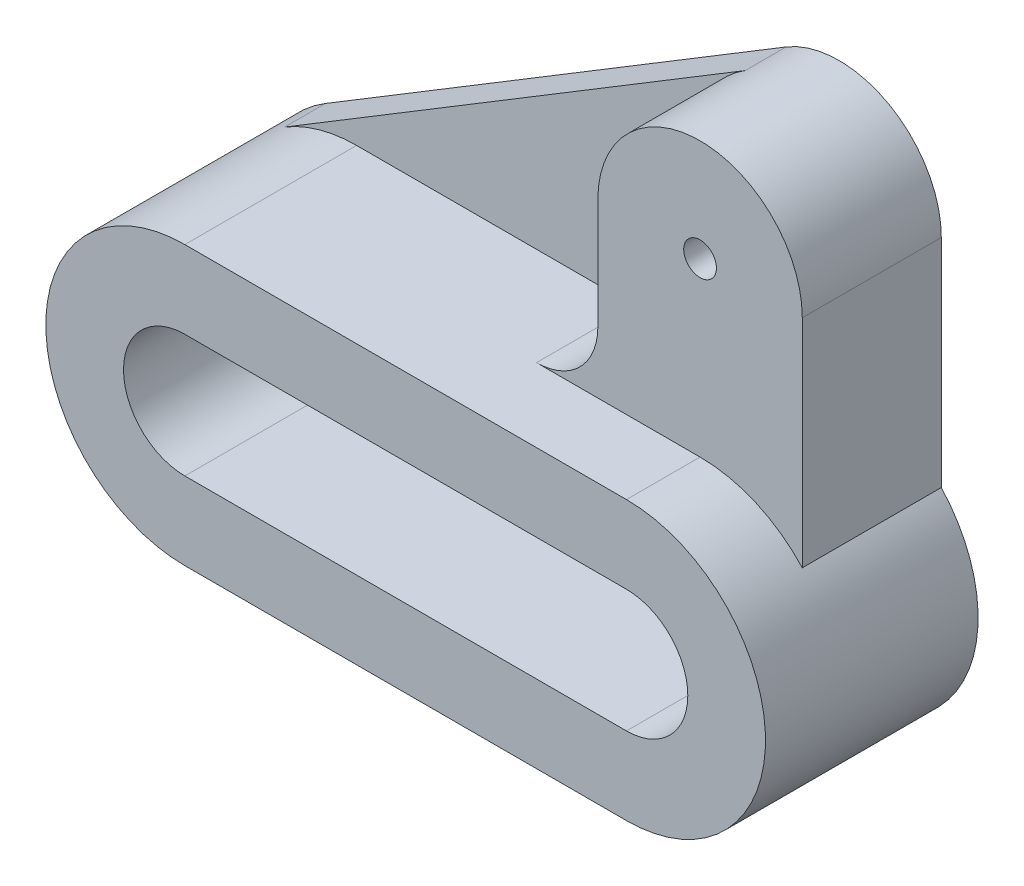
ISO-10303-21;
HEADER;
FILE_DESCRIPTION(('STEP AP214'),'2;1');
FILE_NAME('part.step','',(''),(''),'','','');
FILE_SCHEMA(('AUTOMOTIVE_DESIGN { 1 0 10303 214 1 1 1 1 }'));
ENDSEC;
DATA;
#1=APPLICATION_CONTEXT('core data for automotive mechanical design processes');
#2=APPLICATION_PROTOCOL_DEFINITION('international standard','automotive_design',2000,#1);
#3=PRODUCT_CONTEXT('',#1,'mechanical');
#4=PRODUCT('Part','Part','',(#3));
#5=PRODUCT_RELATED_PRODUCT_CATEGORY('part','',(#4));
#6=PRODUCT_DEFINITION_FORMATION('','',#4);
#7=PRODUCT_DEFINITION_CONTEXT('part definition',#1,'design');
#8=PRODUCT_DEFINITION('design','',#6,#7);
#9=PRODUCT_DEFINITION_SHAPE('','',#8);
#10=(LENGTH_UNIT() NAMED_UNIT(*) SI_UNIT(.MILLI.,.METRE.));
#11=(NAMED_UNIT(*) PLANE_ANGLE_UNIT() SI_UNIT($,.RADIAN.));
#12=(NAMED_UNIT(*) SI_UNIT($,.STERADIAN.) SOLID_ANGLE_UNIT());
#13=UNCERTAINTY_MEASURE_WITH_UNIT(LENGTH_MEASURE(1.E-05),#10,'distance_accuracy_value','');
#14=(GEOMETRIC_REPRESENTATION_CONTEXT(3) GLOBAL_UNCERTAINTY_ASSIGNED_CONTEXT((#13)) GLOBAL_UNIT_ASSIGNED_CONTEXT((#10,
#11,#12)) REPRESENTATION_CONTEXT('',''));
#15=CARTESIAN_POINT('',(0.,0.,0.));
#16=DIRECTION('',(0.,0.,1.));
#17=DIRECTION('',(1.,0.,0.));
#18=AXIS2_PLACEMENT_3D('',#15,#16,#17);
#19=CARTESIAN_POINT('',(54.,0.,52.));
#20=DIRECTION('',(0.,0.,-1.));
#21=DIRECTION('',(-1.,0.,0.));
#22=AXIS2_PLACEMENT_3D('',#19,#20,#21);
#23=CYLINDRICAL_SURFACE('',#22,34.);
#24=DIRECTION('',(0.,0.,-1.));
#25=VECTOR('',#24,1.);
#26=CARTESIAN_POINT('',(54.,-34.,52.));
#27=LINE('',#26,#25);
#28=CARTESIAN_POINT('',(54.,-34.,52.));
#29=VERTEX_POINT('',#28);
#30=CARTESIAN_POINT('',(54.,-34.,0.));
#31=VERTEX_POINT('',#30);
#32=EDGE_CURVE('E231',#29,#31,#27,.T.);
#33=ORIENTED_EDGE('',*,*,#32,.T.);
#34=CARTESIAN_POINT('',(54.,0.,0.));
#35=DIRECTION('',(0.,0.,1.));
#36=DIRECTION('',(1.,0.,0.));
#37=AXIS2_PLACEMENT_3D('',#34,#35,#36);
#38=CIRCLE('',#37,34.);
#39=CARTESIAN_POINT('',(79.,23.0434372436058,0.));
#40=VERTEX_POINT('',#39);
#41=EDGE_CURVE('E216',#31,#40,#38,.T.);
#42=ORIENTED_EDGE('',*,*,#41,.T.);
#43=DIRECTION('',(0.,0.,-1.));
#44=VECTOR('',#43,1.);
#45=CARTESIAN_POINT('',(79.,23.0434372436058,52.));
#46=LINE('',#45,#44);
#47=CARTESIAN_POINT('',(79.,23.0434372436058,34.));
#48=VERTEX_POINT('',#47);
#49=EDGE_CURVE('E168',#48,#40,#46,.T.);
#50=ORIENTED_EDGE('',*,*,#49,.F.);
#51=CARTESIAN_POINT('',(54.,0.,34.));
#52=DIRECTION('',(0.,0.,1.));
#53=DIRECTION('',(1.,0.,0.));
#54=AXIS2_PLACEMENT_3D('',#51,#52,#53);
#55=CIRCLE('',#54,34.);
#56=CARTESIAN_POINT('',(54.,34.,34.));
#57=VERTEX_POINT('',#56);
#58=EDGE_CURVE('E171',#48,#57,#55,.T.);
#59=ORIENTED_EDGE('',*,*,#58,.T.);
#60=DIRECTION('',(0.,0.,-1.));
#61=VECTOR('',#60,1.);
#62=CARTESIAN_POINT('',(54.,34.,52.));
#63=LINE('',#62,#61);
#64=CARTESIAN_POINT('',(54.,34.,52.));
#65=VERTEX_POINT('',#64);
#66=EDGE_CURVE('E234',#65,#57,#63,.T.);
#67=ORIENTED_EDGE('',*,*,#66,.F.);
#68=CARTESIAN_POINT('',(54.,0.,52.));
#69=DIRECTION('',(0.,0.,1.));
#70=DIRECTION('',(1.,0.,0.));
#71=AXIS2_PLACEMENT_3D('',#68,#69,#70);
#72=CIRCLE('',#71,34.);
#73=EDGE_CURVE('E217',#29,#65,#72,.T.);
#74=ORIENTED_EDGE('',*,*,#73,.F.);
#75=EDGE_LOOP('',(#33,#42,#50,#59,#67,#74));
#76=FACE_BOUND('',#75,.T.);
#77=ADVANCED_FACE('F39',(#76),#23,.T.);
#78=CARTESIAN_POINT('',(-54.,34.,52.));
#79=DIRECTION('',(0.,-1.,0.));
#80=DIRECTION('',(1.,0.,0.));
#81=AXIS2_PLACEMENT_3D('',#78,#79,#80);
#82=PLANE('',#81);
#83=DIRECTION('',(-1.,0.,0.));
#84=VECTOR('',#83,1.);
#85=CARTESIAN_POINT('',(-54.,34.,34.));
#86=LINE('',#85,#84);
#87=CARTESIAN_POINT('',(14.,34.,34.));
#88=VERTEX_POINT('',#87);
#89=EDGE_CURVE('E53',#57,#88,#86,.T.);
#90=ORIENTED_EDGE('',*,*,#89,.T.);
#91=DIRECTION('',(0.,0.,1.));
#92=VECTOR('',#91,1.);
#93=CARTESIAN_POINT('',(14.,34.,10.));
#94=LINE('',#93,#92);
#95=CARTESIAN_POINT('',(14.,34.,10.));
#96=VERTEX_POINT('',#95);
#97=EDGE_CURVE('E59',#88,#96,#94,.F.);
#98=ORIENTED_EDGE('',*,*,#97,.T.);
#99=DIRECTION('',(-1.,0.,0.));
#100=VECTOR('',#99,1.);
#101=CARTESIAN_POINT('',(-54.,34.,10.));
#102=LINE('',#101,#100);
#103=CARTESIAN_POINT('',(-54.,34.,10.));
#104=VERTEX_POINT('',#103);
#105=EDGE_CURVE('E249',#96,#104,#102,.T.);
#106=ORIENTED_EDGE('',*,*,#105,.T.);
#107=DIRECTION('',(0.,0.,-1.));
#108=VECTOR('',#107,1.);
#109=CARTESIAN_POINT('',(-54.,34.,52.));
#110=LINE('',#109,#108);
#111=CARTESIAN_POINT('',(-54.,34.,52.));
#112=VERTEX_POINT('',#111);
#113=EDGE_CURVE('E225',#112,#104,#110,.T.);
#114=ORIENTED_EDGE('',*,*,#113,.F.);
#115=DIRECTION('',(-1.,0.,0.));
#116=VECTOR('',#115,1.);
#117=CARTESIAN_POINT('',(-54.,34.,52.));
#118=LINE('',#117,#116);
#119=EDGE_CURVE('E219',#65,#112,#118,.T.);
#120=ORIENTED_EDGE('',*,*,#119,.F.);
#121=ORIENTED_EDGE('',*,*,#66,.T.);
#122=EDGE_LOOP('',(#90,#98,#106,#114,#120,#121));
#123=FACE_BOUND('',#122,.T.);
#124=ADVANCED_FACE('F310',(#123),#82,.F.);
#125=CARTESIAN_POINT('',(-54.,0.,52.));
#126=DIRECTION('',(0.,0.,-1.));
#127=DIRECTION('',(-1.,0.,0.));
#128=AXIS2_PLACEMENT_3D('',#125,#126,#127);
#129=CYLINDRICAL_SURFACE('',#128,34.);
#130=CARTESIAN_POINT('',(-54.,0.,10.));
#131=DIRECTION('',(0.,0.,1.));
#132=DIRECTION('',(1.,0.,0.));
#133=AXIS2_PLACEMENT_3D('',#130,#131,#132);
#134=CIRCLE('',#133,34.);
#135=CARTESIAN_POINT('',(-71.6263298981798,29.0742582763608,10.));
#136=VERTEX_POINT('',#135);
#137=EDGE_CURVE('E285',#104,#136,#134,.T.);
#138=ORIENTED_EDGE('',*,*,#137,.T.);
#139=DIRECTION('',(0.,0.,-1.));
#140=VECTOR('',#139,1.);
#141=CARTESIAN_POINT('',(-71.6263298981798,29.0742582763608,52.));
#142=LINE('',#141,#140);
#143=CARTESIAN_POINT('',(-71.6263298981798,29.0742582763608,0.));
#144=VERTEX_POINT('',#143);
#145=EDGE_CURVE('E277',#144,#136,#142,.F.);
#146=ORIENTED_EDGE('',*,*,#145,.F.);
#147=CARTESIAN_POINT('',(-54.,0.,0.));
#148=DIRECTION('',(0.,0.,1.));
#149=DIRECTION('',(1.,0.,0.));
#150=AXIS2_PLACEMENT_3D('',#147,#148,#149);
#151=CIRCLE('',#150,34.);
#152=CARTESIAN_POINT('',(-54.,-34.,0.));
#153=VERTEX_POINT('',#152);
#154=EDGE_CURVE('E206',#144,#153,#151,.T.);
#155=ORIENTED_EDGE('',*,*,#154,.T.);
#156=DIRECTION('',(0.,0.,-1.));
#157=VECTOR('',#156,1.);
#158=CARTESIAN_POINT('',(-54.,-34.,52.));
#159=LINE('',#158,#157);
#160=CARTESIAN_POINT('',(-54.,-34.,52.));
#161=VERTEX_POINT('',#160);
#162=EDGE_CURVE('E237',#161,#153,#159,.T.);
#163=ORIENTED_EDGE('',*,*,#162,.F.);
#164=CARTESIAN_POINT('',(-54.,0.,52.));
#165=DIRECTION('',(0.,0.,1.));
#166=DIRECTION('',(1.,0.,0.));
#167=AXIS2_PLACEMENT_3D('',#164,#165,#166);
#168=CIRCLE('',#167,34.);
#169=EDGE_CURVE('E215',#112,#161,#168,.T.);
#170=ORIENTED_EDGE('',*,*,#169,.F.);
#171=ORIENTED_EDGE('',*,*,#113,.T.);
#172=EDGE_LOOP('',(#138,#146,#155,#163,#170,#171));
#173=FACE_BOUND('',#172,.T.);
#174=ADVANCED_FACE('F312',(#173),#129,.T.);
#175=CARTESIAN_POINT('',(-54.,-34.,52.));
#176=DIRECTION('',(0.,1.,0.));
#177=DIRECTION('',(-1.,0.,0.));
#178=AXIS2_PLACEMENT_3D('',#175,#176,#177);
#179=PLANE('',#178);
#180=ORIENTED_EDGE('',*,*,#162,.T.);
#181=DIRECTION('',(1.,0.,0.));
#182=VECTOR('',#181,1.);
#183=CARTESIAN_POINT('',(-54.,-34.,0.));
#184=LINE('',#183,#182);
#185=EDGE_CURVE('E223',#153,#31,#184,.T.);
#186=ORIENTED_EDGE('',*,*,#185,.T.);
#187=ORIENTED_EDGE('',*,*,#32,.F.);
#188=DIRECTION('',(1.,0.,0.));
#189=VECTOR('',#188,1.);
#190=CARTESIAN_POINT('',(-54.,-34.,52.));
#191=LINE('',#190,#189);
#192=EDGE_CURVE('E214',#161,#29,#191,.T.);
#193=ORIENTED_EDGE('',*,*,#192,.F.);
#194=EDGE_LOOP('',(#180,#186,#187,#193));
#195=FACE_BOUND('',#194,.T.);
#196=ADVANCED_FACE('F317',(#195),#179,.F.);
#197=CARTESIAN_POINT('',(-54.,0.,52.));
#198=DIRECTION('',(0.,0.,1.));
#199=DIRECTION('',(1.,0.,0.));
#200=AXIS2_PLACEMENT_3D('',#197,#198,#199);
#201=PLANE('',#200);
#202=CARTESIAN_POINT('',(-54.,0.,52.));
#203=DIRECTION('',(0.,0.,1.));
#204=DIRECTION('',(1.,0.,0.));
#205=AXIS2_PLACEMENT_3D('',#202,#203,#204);
#206=CIRCLE('',#205,15.);
#207=CARTESIAN_POINT('',(-54.,15.,52.));
#208=VERTEX_POINT('',#207);
#209=CARTESIAN_POINT('',(-54.,-15.,52.));
#210=VERTEX_POINT('',#209);
#211=EDGE_CURVE('E176',#208,#210,#206,.T.);
#212=ORIENTED_EDGE('',*,*,#211,.F.);
#213=DIRECTION('',(-1.,0.,0.));
#214=VECTOR('',#213,1.);
#215=CARTESIAN_POINT('',(-54.,15.,52.));
#216=LINE('',#215,#214);
#217=CARTESIAN_POINT('',(54.,15.,52.));
#218=VERTEX_POINT('',#217);
#219=EDGE_CURVE('E184',#218,#208,#216,.T.);
#220=ORIENTED_EDGE('',*,*,#219,.F.);
#221=CARTESIAN_POINT('',(54.,0.,52.));
#222=DIRECTION('',(0.,0.,1.));
#223=DIRECTION('',(1.,0.,0.));
#224=AXIS2_PLACEMENT_3D('',#221,#222,#223);
#225=CIRCLE('',#224,15.);
#226=CARTESIAN_POINT('',(54.,-15.,52.));
#227=VERTEX_POINT('',#226);
#228=EDGE_CURVE('E200',#227,#218,#225,.T.);
#229=ORIENTED_EDGE('',*,*,#228,.F.);
#230=DIRECTION('',(1.,0.,0.));
#231=VECTOR('',#230,1.);
#232=CARTESIAN_POINT('',(-54.,-15.,52.));
#233=LINE('',#232,#231);
#234=EDGE_CURVE('E198',#210,#227,#233,.T.);
#235=ORIENTED_EDGE('',*,*,#234,.F.);
#236=EDGE_LOOP('',(#212,#220,#229,#235));
#237=FACE_BOUND('',#236,.T.);
#238=ORIENTED_EDGE('',*,*,#169,.T.);
#239=ORIENTED_EDGE('',*,*,#192,.T.);
#240=ORIENTED_EDGE('',*,*,#73,.T.);
#241=ORIENTED_EDGE('',*,*,#119,.T.);
#242=EDGE_LOOP('',(#238,#239,#240,#241));
#243=FACE_BOUND('',#242,.T.);
#244=ADVANCED_FACE('F321',(#237,#243),#201,.T.);
#245=CARTESIAN_POINT('',(-54.,0.,0.));
#246=DIRECTION('',(0.,0.,1.));
#247=DIRECTION('',(1.,0.,0.));
#248=AXIS2_PLACEMENT_3D('',#245,#246,#247);
#249=PLANE('',#248);
#250=ORIENTED_EDGE('',*,*,#154,.F.);
#251=DIRECTION('',(0.855125243422376,0.518421467593524,0.));
#252=VECTOR('',#251,1.);
#253=CARTESIAN_POINT('',(-71.6263298981798,29.0742582763608,0.));
#254=LINE('',#253,#252);
#255=CARTESIAN_POINT('',(41.0394633101619,97.3781310855594,0.));
#256=VERTEX_POINT('',#255);
#257=EDGE_CURVE('E268',#144,#256,#254,.T.);
#258=ORIENTED_EDGE('',*,*,#257,.T.);
#259=CARTESIAN_POINT('',(54.,76.,0.));
#260=DIRECTION('',(0.,0.,1.));
#261=DIRECTION('',(1.,0.,0.));
#262=AXIS2_PLACEMENT_3D('',#259,#260,#261);
#263=CIRCLE('',#262,25.);
#264=CARTESIAN_POINT('',(79.,76.,0.));
#265=VERTEX_POINT('',#264);
#266=EDGE_CURVE('E260',#265,#256,#263,.T.);
#267=ORIENTED_EDGE('',*,*,#266,.F.);
#268=DIRECTION('',(0.,1.,0.));
#269=VECTOR('',#268,1.);
#270=CARTESIAN_POINT('',(79.,76.,0.));
#271=LINE('',#270,#269);
#272=EDGE_CURVE('E164',#40,#265,#271,.T.);
#273=ORIENTED_EDGE('',*,*,#272,.F.);
#274=ORIENTED_EDGE('',*,*,#41,.F.);
#275=ORIENTED_EDGE('',*,*,#185,.F.);
#276=EDGE_LOOP('',(#250,#258,#267,#273,#274,#275));
#277=FACE_BOUND('',#276,.T.);
#278=CARTESIAN_POINT('',(54.,76.,0.));
#279=DIRECTION('',(0.,0.,1.));
#280=DIRECTION('',(1.,0.,0.));
#281=AXIS2_PLACEMENT_3D('',#278,#279,#280);
#282=CIRCLE('',#281,4.);
#283=CARTESIAN_POINT('',(58.,76.,0.));
#284=VERTEX_POINT('',#283);
#285=EDGE_CURVE('E256',#284,#284,#282,.T.);
#286=ORIENTED_EDGE('',*,*,#285,.T.);
#287=EDGE_LOOP('',(#286));
#288=FACE_BOUND('',#287,.T.);
#289=DIRECTION('',(-1.,0.,0.));
#290=VECTOR('',#289,1.);
#291=CARTESIAN_POINT('',(-54.,15.,0.));
#292=LINE('',#291,#290);
#293=CARTESIAN_POINT('',(54.,15.,0.));
#294=VERTEX_POINT('',#293);
#295=CARTESIAN_POINT('',(-54.,15.,0.));
#296=VERTEX_POINT('',#295);
#297=EDGE_CURVE('E187',#294,#296,#292,.T.);
#298=ORIENTED_EDGE('',*,*,#297,.T.);
#299=CARTESIAN_POINT('',(-54.,0.,0.));
#300=DIRECTION('',(0.,0.,1.));
#301=DIRECTION('',(1.,0.,0.));
#302=AXIS2_PLACEMENT_3D('',#299,#300,#301);
#303=CIRCLE('',#302,15.);
#304=CARTESIAN_POINT('',(-54.,-15.,0.));
#305=VERTEX_POINT('',#304);
#306=EDGE_CURVE('E178',#296,#305,#303,.T.);
#307=ORIENTED_EDGE('',*,*,#306,.T.);
#308=DIRECTION('',(1.,0.,0.));
#309=VECTOR('',#308,1.);
#310=CARTESIAN_POINT('',(-54.,-15.,0.));
#311=LINE('',#310,#309);
#312=CARTESIAN_POINT('',(54.,-15.,0.));
#313=VERTEX_POINT('',#312);
#314=EDGE_CURVE('E181',#305,#313,#311,.T.);
#315=ORIENTED_EDGE('',*,*,#314,.T.);
#316=CARTESIAN_POINT('',(54.,0.,0.));
#317=DIRECTION('',(0.,0.,1.));
#318=DIRECTION('',(1.,0.,0.));
#319=AXIS2_PLACEMENT_3D('',#316,#317,#318);
#320=CIRCLE('',#319,15.);
#321=EDGE_CURVE('E190',#313,#294,#320,.T.);
#322=ORIENTED_EDGE('',*,*,#321,.T.);
#323=EDGE_LOOP('',(#298,#307,#315,#322));
#324=FACE_BOUND('',#323,.T.);
#325=ADVANCED_FACE('F264',(#277,#288,#324),#249,.F.);
#326=CARTESIAN_POINT('',(-54.,0.,0.));
#327=DIRECTION('',(0.,0.,1.));
#328=DIRECTION('',(1.,0.,0.));
#329=AXIS2_PLACEMENT_3D('',#326,#327,#328);
#330=CYLINDRICAL_SURFACE('',#329,15.);
#331=ORIENTED_EDGE('',*,*,#211,.T.);
#332=DIRECTION('',(0.,0.,1.));
#333=VECTOR('',#332,1.);
#334=CARTESIAN_POINT('',(-54.,-15.,0.));
#335=LINE('',#334,#333);
#336=EDGE_CURVE('E195',#305,#210,#335,.T.);
#337=ORIENTED_EDGE('',*,*,#336,.F.);
#338=ORIENTED_EDGE('',*,*,#306,.F.);
#339=DIRECTION('',(0.,0.,1.));
#340=VECTOR('',#339,1.);
#341=CARTESIAN_POINT('',(-54.,15.,0.));
#342=LINE('',#341,#340);
#343=EDGE_CURVE('E204',#296,#208,#342,.T.);
#344=ORIENTED_EDGE('',*,*,#343,.T.);
#345=EDGE_LOOP('',(#331,#337,#338,#344));
#346=FACE_BOUND('',#345,.T.);
#347=ADVANCED_FACE('F339',(#346),#330,.F.);
#348=CARTESIAN_POINT('',(-54.,15.,0.));
#349=DIRECTION('',(0.,1.,0.));
#350=DIRECTION('',(-1.,0.,0.));
#351=AXIS2_PLACEMENT_3D('',#348,#349,#350);
#352=PLANE('',#351);
#353=ORIENTED_EDGE('',*,*,#219,.T.);
#354=ORIENTED_EDGE('',*,*,#343,.F.);
#355=ORIENTED_EDGE('',*,*,#297,.F.);
#356=DIRECTION('',(0.,0.,1.));
#357=VECTOR('',#356,1.);
#358=CARTESIAN_POINT('',(54.,15.,0.));
#359=LINE('',#358,#357);
#360=EDGE_CURVE('E210',#294,#218,#359,.T.);
#361=ORIENTED_EDGE('',*,*,#360,.T.);
#362=EDGE_LOOP('',(#353,#354,#355,#361));
#363=FACE_BOUND('',#362,.T.);
#364=ADVANCED_FACE('F345',(#363),#352,.F.);
#365=CARTESIAN_POINT('',(54.,0.,0.));
#366=DIRECTION('',(0.,0.,1.));
#367=DIRECTION('',(1.,0.,0.));
#368=AXIS2_PLACEMENT_3D('',#365,#366,#367);
#369=CYLINDRICAL_SURFACE('',#368,15.);
#370=ORIENTED_EDGE('',*,*,#228,.T.);
#371=ORIENTED_EDGE('',*,*,#360,.F.);
#372=ORIENTED_EDGE('',*,*,#321,.F.);
#373=DIRECTION('',(0.,0.,1.));
#374=VECTOR('',#373,1.);
#375=CARTESIAN_POINT('',(54.,-15.,0.));
#376=LINE('',#375,#374);
#377=EDGE_CURVE('E207',#313,#227,#376,.T.);
#378=ORIENTED_EDGE('',*,*,#377,.T.);
#379=EDGE_LOOP('',(#370,#371,#372,#378));
#380=FACE_BOUND('',#379,.T.);
#381=ADVANCED_FACE('F305',(#380),#369,.F.);
#382=CARTESIAN_POINT('',(-54.,-15.,0.));
#383=DIRECTION('',(0.,-1.,0.));
#384=DIRECTION('',(1.,0.,0.));
#385=AXIS2_PLACEMENT_3D('',#382,#383,#384);
#386=PLANE('',#385);
#387=ORIENTED_EDGE('',*,*,#234,.T.);
#388=ORIENTED_EDGE('',*,*,#377,.F.);
#389=ORIENTED_EDGE('',*,*,#314,.F.);
#390=ORIENTED_EDGE('',*,*,#336,.T.);
#391=EDGE_LOOP('',(#387,#388,#389,#390));
#392=FACE_BOUND('',#391,.T.);
#393=ADVANCED_FACE('F293',(#392),#386,.F.);
#394=CARTESIAN_POINT('',(54.,76.,34.));
#395=DIRECTION('',(0.,0.,1.));
#396=DIRECTION('',(1.,0.,0.));
#397=AXIS2_PLACEMENT_3D('',#394,#395,#396);
#398=PLANE('',#397);
#399=CARTESIAN_POINT('',(54.,76.,34.));
#400=DIRECTION('',(0.,0.,1.));
#401=DIRECTION('',(1.,0.,0.));
#402=AXIS2_PLACEMENT_3D('',#399,#400,#401);
#403=CIRCLE('',#402,4.);
#404=CARTESIAN_POINT('',(58.,76.,34.));
#405=VERTEX_POINT('',#404);
#406=EDGE_CURVE('E282',#405,#405,#403,.T.);
#407=ORIENTED_EDGE('',*,*,#406,.F.);
#408=EDGE_LOOP('',(#407));
#409=FACE_BOUND('',#408,.T.);
#410=ORIENTED_EDGE('',*,*,#58,.F.);
#411=DIRECTION('',(0.,1.,0.));
#412=VECTOR('',#411,1.);
#413=CARTESIAN_POINT('',(79.,76.,34.));
#414=LINE('',#413,#412);
#415=CARTESIAN_POINT('',(79.,76.,34.));
#416=VERTEX_POINT('',#415);
#417=EDGE_CURVE('E156',#48,#416,#414,.T.);
#418=ORIENTED_EDGE('',*,*,#417,.T.);
#419=CARTESIAN_POINT('',(54.,76.,34.));
#420=DIRECTION('',(0.,0.,1.));
#421=DIRECTION('',(1.,0.,0.));
#422=AXIS2_PLACEMENT_3D('',#419,#420,#421);
#423=CIRCLE('',#422,25.);
#424=CARTESIAN_POINT('',(29.,76.,34.));
#425=VERTEX_POINT('',#424);
#426=EDGE_CURVE('E160',#416,#425,#423,.T.);
#427=ORIENTED_EDGE('',*,*,#426,.T.);
#428=DIRECTION('',(0.,-1.,0.));
#429=VECTOR('',#428,1.);
#430=CARTESIAN_POINT('',(29.,76.,34.));
#431=LINE('',#430,#429);
#432=CARTESIAN_POINT('',(29.,49.,34.));
#433=VERTEX_POINT('',#432);
#434=EDGE_CURVE('E148',#425,#433,#431,.T.);
#435=ORIENTED_EDGE('',*,*,#434,.T.);
#436=CARTESIAN_POINT('',(14.,49.,34.));
#437=DIRECTION('',(0.,0.,1.));
#438=DIRECTION('',(1.,0.,0.));
#439=AXIS2_PLACEMENT_3D('',#436,#437,#438);
#440=CIRCLE('',#439,15.);
#441=EDGE_CURVE('E11',#433,#88,#440,.F.);
#442=ORIENTED_EDGE('',*,*,#441,.T.);
#443=ORIENTED_EDGE('',*,*,#89,.F.);
#444=EDGE_LOOP('',(#410,#418,#427,#435,#442,#443));
#445=FACE_BOUND('',#444,.T.);
#446=ADVANCED_FACE('F161',(#409,#445),#398,.T.);
#447=CARTESIAN_POINT('',(29.,18.0315919180991,34.));
#448=DIRECTION('',(1.,0.,0.));
#449=DIRECTION('',(0.,0.,-1.));
#450=AXIS2_PLACEMENT_3D('',#447,#448,#449);
#451=PLANE('',#450);
#452=DIRECTION('',(0.,-1.,0.));
#453=VECTOR('',#452,1.);
#454=CARTESIAN_POINT('',(29.,18.0315919180991,10.));
#455=LINE('',#454,#453);
#456=CARTESIAN_POINT('',(29.,76.,10.));
#457=VERTEX_POINT('',#456);
#458=CARTESIAN_POINT('',(29.,49.,10.));
#459=VERTEX_POINT('',#458);
#460=EDGE_CURVE('E242',#457,#459,#455,.T.);
#461=ORIENTED_EDGE('',*,*,#460,.T.);
#462=DIRECTION('',(0.,0.,1.));
#463=VECTOR('',#462,1.);
#464=CARTESIAN_POINT('',(29.,49.,34.));
#465=LINE('',#464,#463);
#466=EDGE_CURVE('E152',#459,#433,#465,.T.);
#467=ORIENTED_EDGE('',*,*,#466,.T.);
#468=ORIENTED_EDGE('',*,*,#434,.F.);
#469=DIRECTION('',(0.,0.,-1.));
#470=VECTOR('',#469,1.);
#471=CARTESIAN_POINT('',(29.,76.,34.));
#472=LINE('',#471,#470);
#473=EDGE_CURVE('E151',#425,#457,#472,.T.);
#474=ORIENTED_EDGE('',*,*,#473,.T.);
#475=EDGE_LOOP('',(#461,#467,#468,#474));
#476=FACE_BOUND('',#475,.T.);
#477=ADVANCED_FACE('F149',(#476),#451,.F.);
#478=CARTESIAN_POINT('',(79.,76.,34.));
#479=DIRECTION('',(-1.,0.,0.));
#480=DIRECTION('',(0.,0.,1.));
#481=AXIS2_PLACEMENT_3D('',#478,#479,#480);
#482=PLANE('',#481);
#483=ORIENTED_EDGE('',*,*,#49,.T.);
#484=ORIENTED_EDGE('',*,*,#272,.T.);
#485=DIRECTION('',(0.,0.,-1.));
#486=VECTOR('',#485,1.);
#487=CARTESIAN_POINT('',(79.,76.,34.));
#488=LINE('',#487,#486);
#489=EDGE_CURVE('E173',#416,#265,#488,.T.);
#490=ORIENTED_EDGE('',*,*,#489,.F.);
#491=ORIENTED_EDGE('',*,*,#417,.F.);
#492=EDGE_LOOP('',(#483,#484,#490,#491));
#493=FACE_BOUND('',#492,.T.);
#494=ADVANCED_FACE('F251',(#493),#482,.F.);
#495=CARTESIAN_POINT('',(54.,76.,34.));
#496=DIRECTION('',(0.,0.,-1.));
#497=DIRECTION('',(-1.,0.,0.));
#498=AXIS2_PLACEMENT_3D('',#495,#496,#497);
#499=CYLINDRICAL_SURFACE('',#498,25.);
#500=ORIENTED_EDGE('',*,*,#489,.T.);
#501=ORIENTED_EDGE('',*,*,#266,.T.);
#502=DIRECTION('',(0.,0.,-1.));
#503=VECTOR('',#502,1.);
#504=CARTESIAN_POINT('',(41.0394633101619,97.3781310855594,34.));
#505=LINE('',#504,#503);
#506=CARTESIAN_POINT('',(41.0394633101619,97.3781310855594,10.));
#507=VERTEX_POINT('',#506);
#508=EDGE_CURVE('E239',#256,#507,#505,.F.);
#509=ORIENTED_EDGE('',*,*,#508,.T.);
#510=CARTESIAN_POINT('',(54.,76.,10.));
#511=DIRECTION('',(0.,0.,1.));
#512=DIRECTION('',(1.,0.,0.));
#513=AXIS2_PLACEMENT_3D('',#510,#511,#512);
#514=CIRCLE('',#513,25.);
#515=EDGE_CURVE('E166',#507,#457,#514,.T.);
#516=ORIENTED_EDGE('',*,*,#515,.T.);
#517=ORIENTED_EDGE('',*,*,#473,.F.);
#518=ORIENTED_EDGE('',*,*,#426,.F.);
#519=EDGE_LOOP('',(#500,#501,#509,#516,#517,#518));
#520=FACE_BOUND('',#519,.T.);
#521=ADVANCED_FACE('F170',(#520),#499,.T.);
#522=CARTESIAN_POINT('',(54.,76.,0.));
#523=DIRECTION('',(0.,0.,1.));
#524=DIRECTION('',(1.,0.,0.));
#525=AXIS2_PLACEMENT_3D('',#522,#523,#524);
#526=CYLINDRICAL_SURFACE('',#525,4.);
#527=ORIENTED_EDGE('',*,*,#406,.T.);
#528=EDGE_LOOP('',(#527));
#529=FACE_BOUND('',#528,.T.);
#530=ORIENTED_EDGE('',*,*,#285,.F.);
#531=EDGE_LOOP('',(#530));
#532=FACE_BOUND('',#531,.T.);
#533=ADVANCED_FACE('F292',(#529,#532),#526,.F.);
#534=CARTESIAN_POINT('',(-71.6263298981798,29.0742582763608,0.));
#535=DIRECTION('',(0.518421467593524,-0.855125243422376,0.));
#536=DIRECTION('',(0.855125243422376,0.518421467593524,0.));
#537=AXIS2_PLACEMENT_3D('',#534,#535,#536);
#538=PLANE('',#537);
#539=ORIENTED_EDGE('',*,*,#257,.F.);
#540=ORIENTED_EDGE('',*,*,#145,.T.);
#541=DIRECTION('',(0.855125243422376,0.518421467593524,0.));
#542=VECTOR('',#541,1.);
#543=CARTESIAN_POINT('',(-71.6263298981798,29.0742582763608,10.));
#544=LINE('',#543,#542);
#545=EDGE_CURVE('E274',#136,#507,#544,.T.);
#546=ORIENTED_EDGE('',*,*,#545,.T.);
#547=ORIENTED_EDGE('',*,*,#508,.F.);
#548=EDGE_LOOP('',(#539,#540,#546,#547));
#549=FACE_BOUND('',#548,.T.);
#550=ADVANCED_FACE('F275',(#549),#538,.F.);
#551=CARTESIAN_POINT('',(0.,33.5,10.));
#552=DIRECTION('',(0.,0.,1.));
#553=DIRECTION('',(1.,0.,0.));
#554=AXIS2_PLACEMENT_3D('',#551,#552,#553);
#555=PLANE('',#554);
#556=ORIENTED_EDGE('',*,*,#105,.F.);
#557=CARTESIAN_POINT('',(14.,49.,10.));
#558=DIRECTION('',(0.,0.,1.));
#559=DIRECTION('',(1.,0.,0.));
#560=AXIS2_PLACEMENT_3D('',#557,#558,#559);
#561=CIRCLE('',#560,15.);
#562=EDGE_CURVE('E50',#96,#459,#561,.T.);
#563=ORIENTED_EDGE('',*,*,#562,.T.);
#564=ORIENTED_EDGE('',*,*,#460,.F.);
#565=ORIENTED_EDGE('',*,*,#515,.F.);
#566=ORIENTED_EDGE('',*,*,#545,.F.);
#567=ORIENTED_EDGE('',*,*,#137,.F.);
#568=EDGE_LOOP('',(#556,#563,#564,#565,#566,#567));
#569=FACE_BOUND('',#568,.T.);
#570=ADVANCED_FACE('F244',(#569),#555,.T.);
#571=CARTESIAN_POINT('',(14.,49.,34.));
#572=DIRECTION('',(0.,0.,-1.));
#573=DIRECTION('',(-1.,0.,0.));
#574=AXIS2_PLACEMENT_3D('',#571,#572,#573);
#575=CYLINDRICAL_SURFACE('',#574,15.);
#576=ORIENTED_EDGE('',*,*,#562,.F.);
#577=ORIENTED_EDGE('',*,*,#97,.F.);
#578=ORIENTED_EDGE('',*,*,#441,.F.);
#579=ORIENTED_EDGE('',*,*,#466,.F.);
#580=EDGE_LOOP('',(#576,#577,#578,#579));
#581=FACE_BOUND('',#580,.T.);
#582=ADVANCED_FACE('F41',(#581),#575,.F.);
#583=CLOSED_SHELL('',(#77,#124,#174,#196,#244,#325,#347,#364,#381,#393,#446,#477,#494,#521,#533,
#550,#570,#582));
#584=MANIFOLD_SOLID_BREP('B2',#583);
#585=ADVANCED_BREP_SHAPE_REPRESENTATION('',(#18,#584),#14);
#586=SHAPE_DEFINITION_REPRESENTATION(#9,#585);
ENDSEC;
END-ISO-10303-21;
